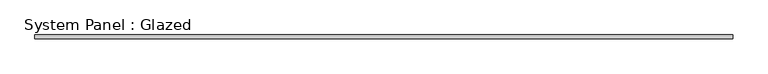
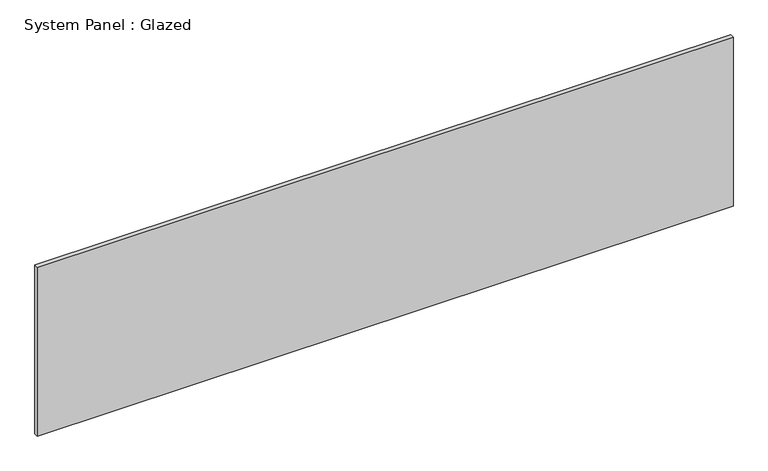
"""IFC4 building model written with IfcOpenShell, lengths in millimetres: plate geometry, System Panel : Glazed."""

from ifc_helpers import new_model, si_unit, origin, origin_with_axes, place, context, project, spatial, polyline, outline, extrude, source, transform, mapped, element, save


def system_panel_glazed_2980b8bc(model_context):
    return source(origin(), model_context, "Body", "SweptSolid", [
        extrude(outline(polyline([(2375.0739558, 19.05), (-2375.0739558, 19.05), (-2375.0739558, 44.45), (2375.0739558, 44.45), (2375.0739558, 19.05)])), origin_with_axes(), (0.0, 0.0, 1.0), 1219.2),
    ])


if __name__ == "__main__":
    model = new_model("IFC4")
    model_context = context("Model", 3, world=origin())
    ifc_project = project(units=[si_unit("LENGTHUNIT", "METRE", prefix="MILLI")], contexts=[model_context])
    site = spatial("IfcSite", under=ifc_project)
    building = spatial("IfcBuilding", under=site)
    placement = place(None, origin())
    system_panel_glazed_shape = system_panel_glazed_2980b8bc(model_context)
    element("IfcPlate", 1, ObjectType="System Panel : Glazed", at=placement, inside=building, context=model_context, shape_type="MappedRepresentation", body=[
        mapped(system_panel_glazed_shape, transform((0.0, 0.0, 0.0), x_axis=(1.0, 0.0, 0.0), y_axis=(0.0, 1.0, 0.0), z_axis=(0.0, 0.0, 1.0))),
    ])
    save(model, "model.ifc")

# Revit data of these elements
# Type "System Panel : Glazed"
#   Construction Type Id = "GSP4R"
#   Analytic Construction = "1/8 in Pilkington single glazing"
#   Visual Light Transmittance = 0.9
#   Solar Heat Gain Coefficient = 0.86
#   Heat Transfer Coefficient (U) = 1.18115 BTU/(h·ft²·°F)
# Element 1 (IfcPlate, "System Panel : Glazed")
#   Materials on its faces: "Glass"
# Materials
#   "Glass": class "Glass", colour RGB 0 128 192, transparency 0.75, Description = "Soda Lime Glass", Cost = 0
